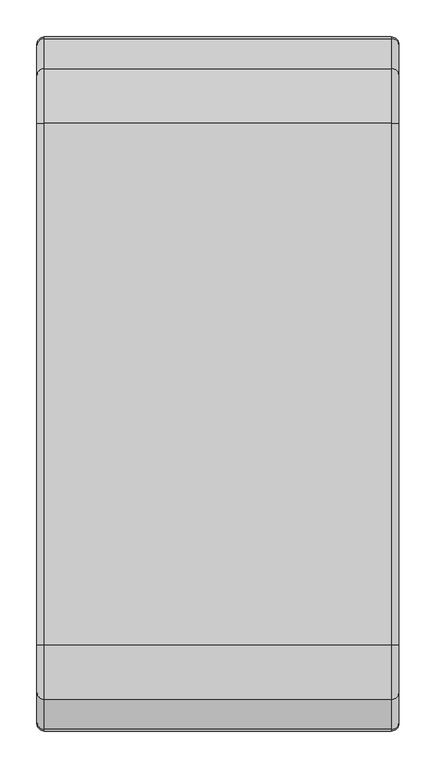
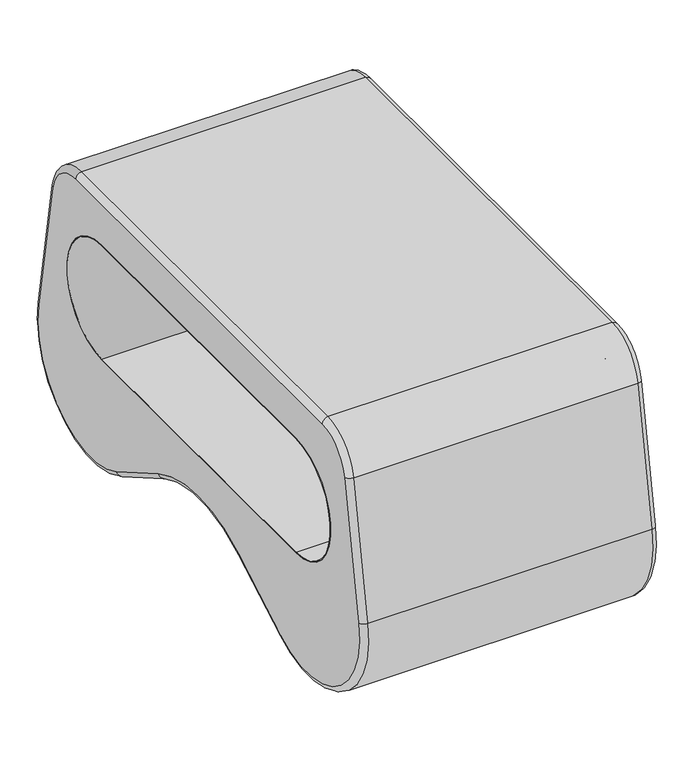
"""IFC4 building model written with IfcOpenShell, lengths in millimetres: furniture geometry."""

from ifc_helpers import new_model, si_unit, point, frame, origin, place, context, project, spatial, polyline, circle_curve, ellipse_curve, trimmed, source, transform, mapped, element, save
from ifc_brep_helpers import plane_surface, cylinder_surface, revolved_surface, advanced_brep


def furniture_2dca108f(model_context):
    return source(origin(), model_context, "Body", "AdvancedBrep", [
        advanced_brep(
        [(245.0, 417.1236557, 416.2871315), (245.0, 353.1111517, 470.0), (245.0, -353.1111517, 470.0), (245.0, -417.1236557, 416.2871315), (245.0, -457.721163, 186.0472267), (245.0, -235.0, 30.0961894), (245.0, -115.0, 99.3782217), (245.0, 115.0, 99.3782217), (245.0, 235.0, 30.0961894), (245.0, 457.721163, 186.0472267), (245.0, 278.278004, 200.0), (245.0, -278.278004, 200.0), (245.0, -278.278004, 400.0), (245.0, 278.278004, 400.0), (-245.0, 353.1111517, 470.0), (-245.0, 417.1236557, 416.2871315), (-245.0, 457.721163, 186.0472267), (-245.0, 235.0, 30.0961894), (-245.0, 115.0, 99.3782217), (-245.0, -115.0, 99.3782217), (-245.0, -235.0, 30.0961894), (-245.0, -457.721163, 186.0472267), (-245.0, -417.1236557, 416.2871315), (-245.0, -353.1111517, 470.0), (-245.0, 278.278004, 200.0), (-245.0, 278.278004, 400.0), (-245.0, -278.278004, 400.0), (-245.0, -278.278004, 200.0), (-235.0, 353.1111517, 480.0), (-235.0, -353.1111517, 480.0), (235.0, -353.1111517, 480.0), (235.0, 353.1111517, 480.0), (-235.0, -426.9717332, 418.0236133), (235.0000137, -426.9717332, 418.0236133), (-235.0, -467.5692405, 187.7837084), (235.0, -467.5692405, 187.7837084), (-235.0, -230.0, 21.4359354), (235.0000033, -230.0, 21.4359354), (-235.0, -110.0, 90.7179677), (235.0, -110.0, 90.7179677), (-235.0, 110.0, 90.7179677), (235.000004, 110.0, 90.7179677), (-235.0, 230.0, 21.4359354), (235.0, 230.0, 21.4359354), (-235.0, 467.5692405, 187.7837084), (235.0000035, 467.5692405, 187.7837084), (-235.0, 426.9717332, 418.0236133), (235.0000138, 426.9717332, 418.0236133), (244.0, 278.278004, 200.0), (-244.0, 278.278004, 200.0), (-244.0, -278.278004, 200.0), (244.0000012, -278.278004, 200.0), (-244.0, -278.278004, 400.0), (244.0000005, -278.278004, 400.0), (-244.0, 278.278004, 400.0), (244.0000012, 278.278004, 400.0)],
        [
            (0, 1, circle_curve(frame((245.0, 353.1111517, 405.0), z_axis=(1.0, 0.0, 0.0), x_axis=(0.0, 0.9848077530122095, 0.1736481776669226)), 65.0)),
            (1, 2),
            (2, 3, circle_curve(frame((245.0, -353.1111517, 405.0), z_axis=(1.0, 0.0, 0.0), x_axis=(0.0, 0.0, 1.0)), 65.0)),
            (3, 4),
            (4, 5, circle_curve(frame((245.0, -310.0, 160.0), z_axis=(1.0, 0.0, 0.0), x_axis=(0.0, -0.9848077530122084, 0.17364817766692853)), 150.0)),
            (5, 6),
            (6, 7, circle_curve(frame((245.0, 0.0, -99.8076211), z_axis=(-1.0, 0.0, 0.0), x_axis=(0.0, -0.4999999999999878, 0.8660254037844457)), 230.0)),
            (7, 8),
            (8, 9, circle_curve(frame((245.0, 310.0, 160.0), z_axis=(1.0, 0.0, 0.0), x_axis=(0.0, -0.5000000000000022, -0.8660254037844374)), 150.0)),
            (9, 0),
            (10, 11),
            (11, 12, circle_curve(frame((245.0, -278.278004, 300.0), z_axis=(-1.0, 0.0, 0.0), x_axis=(0.0, 1.0, 0.0)), 100.0)),
            (12, 13),
            (13, 10, circle_curve(frame((245.0, 278.278004, 300.0), z_axis=(-1.0, 0.0, 0.0), x_axis=(0.0, -1.0, 0.0)), 100.0)),
            (14, 15, circle_curve(frame((-245.0, 353.1111517, 405.0), z_axis=(-1.0, 0.0, 0.0), x_axis=(0.0, 0.9848077530122092, 0.17364817766692348)), 65.0)),
            (15, 16),
            (16, 17, circle_curve(frame((-245.0, 310.0, 160.0), z_axis=(-1.0, 0.0, 0.0), x_axis=(0.0, -0.5000000000000022, -0.8660254037844374)), 150.0)),
            (17, 18),
            (18, 19, circle_curve(frame((-245.0, 0.0, -99.8076211), z_axis=(1.0, 0.0, 0.0), x_axis=(0.0, -0.4999999999999878, 0.8660254037844457)), 230.0)),
            (19, 20),
            (20, 21, circle_curve(frame((-245.0, -310.0, 160.0), z_axis=(-1.0, 0.0, 0.0), x_axis=(0.0, -0.9848077530122084, 0.17364817766692853)), 150.0)),
            (21, 22),
            (22, 23, circle_curve(frame((-245.0, -353.1111517, 405.0), z_axis=(-1.0, 0.0, 0.0), x_axis=(0.0, 0.0, 1.0)), 65.0)),
            (23, 14),
            (24, 25, circle_curve(frame((-245.0, 278.278004, 300.0), z_axis=(1.0, 0.0, 0.0), x_axis=(0.0, -1.0, 0.0)), 100.0)),
            (25, 26),
            (26, 27, circle_curve(frame((-245.0, -278.278004, 300.0), z_axis=(1.0, 0.0, 0.0), x_axis=(0.0, 1.0, 0.0)), 100.0)),
            (27, 24),
            (28, 29),
            (29, 30),
            (30, 31),
            (31, 28),
            (29, 32, circle_curve(frame((-235.0, -353.1111517, 405.0), z_axis=(1.0, 0.0, 0.0), x_axis=(0.0, 1.0, 0.0)), 75.0)),
            (32, 33),
            (33, 30, circle_curve(frame((235.0, -353.1111517, 405.0), z_axis=(-1.0, 0.0, 0.0), x_axis=(0.0, 1.0, 0.0)), 75.0)),
            (32, 34),
            (34, 35),
            (35, 33),
            (34, 36, circle_curve(frame((-235.0, -310.0, 160.0), z_axis=(1.0, 0.0, 0.0), x_axis=(0.0, 1.0, 0.0)), 160.0)),
            (36, 37),
            (37, 35, circle_curve(frame((235.0, -310.0, 160.0), z_axis=(-1.0, 0.0, 0.0), x_axis=(0.0, 1.0, 0.0)), 160.0)),
            (36, 38),
            (38, 39),
            (39, 37),
            (38, 40, circle_curve(frame((-235.0, 0.0, -99.8076211), z_axis=(-1.0, 0.0, 0.0), x_axis=(0.0, -1.0, 0.0)), 220.0)),
            (40, 41),
            (41, 39, circle_curve(frame((235.0, 0.0, -99.8076211), z_axis=(1.0, 0.0, 0.0), x_axis=(0.0, -1.0, 0.0)), 220.0)),
            (40, 42),
            (42, 43),
            (43, 41),
            (42, 44, circle_curve(frame((-235.0, 310.0, 160.0), z_axis=(1.0, 0.0, 0.0), x_axis=(0.0, -1.0, 0.0)), 160.0)),
            (44, 45),
            (45, 43, circle_curve(frame((235.0, 310.0, 160.0), z_axis=(-1.0, 0.0, 0.0), x_axis=(0.0, -1.0, 0.0)), 160.0)),
            (44, 46),
            (46, 47),
            (47, 45),
            (46, 28, circle_curve(frame((-235.0, 353.1111517, 405.0), z_axis=(1.0, 0.0, 0.0), x_axis=(0.0, -1.0, 0.0)), 75.0)),
            (31, 47, circle_curve(frame((235.0, 353.1111517, 405.0), z_axis=(-1.0, 0.0, 0.0), x_axis=(0.0, -1.0, 0.0)), 75.0)),
            (10, 48),
            (48, 49),
            (49, 24),
            (27, 50),
            (50, 51),
            (51, 11),
            (26, 52),
            (52, 53),
            (53, 12),
            (25, 54),
            (54, 55),
            (55, 13),
            (14, 28, circle_curve(frame((-235.0, 353.1111517, 470.0), z_axis=(0.0, 1.0, 0.0), x_axis=(-1.0, 0.0, 0.0)), 10.0)),
            (46, 15, circle_curve(frame((-235.0, 417.1236557, 416.2871315), z_axis=(0.0, -0.17364817766692348, 0.9848077530122092), x_axis=(-1.0, 0.0, 0.0)), 10.0)),
            (23, 29, circle_curve(frame((-235.0, -353.1111517, 470.0), z_axis=(0.0, 1.0, 0.0), x_axis=(-1.0, 0.0, 0.0)), 10.0)),
            (22, 32, circle_curve(frame((-235.0, -417.1236557, 416.2871315), z_axis=(0.0, 0.17364817766692897, 0.9848077530122084), x_axis=(-1.0, 0.0, 0.0)), 10.0)),
            (21, 34, circle_curve(frame((-235.0, -457.721163, 186.0472267), z_axis=(0.0, 0.1736481776669289, 0.9848077530122084), x_axis=(-1.0, 0.0, 0.0)), 10.0)),
            (20, 36, circle_curve(frame((-235.0, -235.0, 30.0961894), z_axis=(0.0, -0.8660254037844488, -0.4999999999999824), x_axis=(-1.0, 0.0, 0.0)), 10.0)),
            (19, 38, circle_curve(frame((-235.0, -115.0, 99.3782217), z_axis=(0.0, -0.8660254037844457, -0.4999999999999879), x_axis=(-1.0, 0.0, 0.0)), 10.0)),
            (18, 40, circle_curve(frame((-235.0, 115.0, 99.3782217), z_axis=(0.0, -0.8660254037844375, 0.500000000000002), x_axis=(-1.0, 0.0, 0.0)), 10.0)),
            (17, 42, circle_curve(frame((-235.0, 235.0, 30.0961894), z_axis=(0.0, -0.8660254037844374, 0.5000000000000023), x_axis=(-1.0, 0.0, 0.0)), 10.0)),
            (16, 44, circle_curve(frame((-235.0, 457.721163, 186.0472267), z_axis=(0.0, 0.1736481776669226, -0.9848077530122095), x_axis=(-1.0, 0.0, 0.0)), 10.0)),
            (31, 1, circle_curve(frame((235.0, 353.1111517, 470.0), z_axis=(0.0, 1.0, 0.0), x_axis=(1.0, 0.0, 0.0)), 10.0)),
            (0, 47, circle_curve(frame((235.0, 417.1236557, 416.2871315), z_axis=(0.0, -0.1736481776669226, 0.9848077530122095), x_axis=(1.0, 0.0, 0.0)), 10.0)),
            (30, 2, circle_curve(frame((235.0, -353.1111517, 470.0), z_axis=(0.0, 1.0, 0.0), x_axis=(1.0, 0.0, 0.0)), 10.0)),
            (33, 3, circle_curve(frame((235.0, -417.1236557, 416.2871315), z_axis=(0.0, 0.1736481776669292, 0.9848077530122084), x_axis=(1.0, 0.0, 0.0)), 10.0)),
            (35, 4, circle_curve(frame((235.0, -457.721163, 186.0472267), z_axis=(0.0, 0.1736481776669289, 0.9848077530122084), x_axis=(1.0, 0.0, 0.0)), 10.0)),
            (37, 5, circle_curve(frame((235.0, -235.0, 30.0961894), z_axis=(0.0, -0.8660254037844488, -0.4999999999999824), x_axis=(1.0, 0.0, 0.0)), 10.0)),
            (39, 6, circle_curve(frame((235.0, -115.0, 99.3782217), z_axis=(0.0, -0.8660254037844457, -0.4999999999999879), x_axis=(1.0, 0.0, 0.0)), 10.0)),
            (41, 7, circle_curve(frame((235.0, 115.0, 99.3782217), z_axis=(0.0, -0.8660254037844375, 0.5000000000000022), x_axis=(1.0, 0.0, 0.0)), 10.0)),
            (43, 8, circle_curve(frame((235.0, 235.0, 30.0961894), z_axis=(0.0, -0.8660254037844375, 0.5000000000000022), x_axis=(1.0, 0.0, 0.0)), 10.0)),
            (45, 9, circle_curve(frame((235.0, 457.721163, 186.0472267), z_axis=(0.0, 0.1736481776669226, -0.9848077530122095), x_axis=(1.0, 0.0, 0.0)), 10.0)),
        ],
        [
            plane_surface(frame((245.0, 0.0, 480.0), z_axis=(1.0, 0.0, 0.0), x_axis=(0.0, -1.0, 0.0))),
            plane_surface(frame((-245.0, 0.0, 480.0), z_axis=(-1.0, 0.0, 0.0), x_axis=(0.0, 1.0, 0.0))),
            plane_surface(frame((245.0, 353.1111517, 480.0), z_axis=(0.0, 0.0, 1.0), x_axis=(-1.0, 0.0, 0.0))),
            cylinder_surface(frame((-245.0, -353.1111517, 405.0), z_axis=(1.0, 0.0, 0.0), x_axis=(0.0, 1.0, 0.0)), 75.0),
            plane_surface(frame((245.0, -426.9717332, 418.0236133), z_axis=(0.0, -0.9848077530122084, 0.17364817766692886), x_axis=(-1.0, 0.0, 0.0))),
            cylinder_surface(frame((-245.0, -310.0, 160.0), z_axis=(1.0, 0.0, 0.0), x_axis=(0.0, 1.0, 0.0)), 160.0),
            plane_surface(frame((245.0, -230.0, 21.4359354), z_axis=(0.0, 0.4999999999999879, -0.8660254037844457), x_axis=(-1.0, 0.0, 0.0))),
            revolved_surface(polyline([(-235.0, -220.0, -99.8076211), (235.000004, -220.0, -99.8076211)]), (-245.0, 0.0, -99.8076211), (-1.0, 0.0, 0.0)),
            plane_surface(frame((245.0, 110.0, 90.7179677), z_axis=(0.0, -0.5000000000000021, -0.8660254037844375), x_axis=(-1.0, 0.0, 0.0))),
            cylinder_surface(frame((-245.0, 310.0, 160.0), z_axis=(1.0, 0.0, 0.0), x_axis=(0.0, -1.0, 0.0)), 160.0),
            plane_surface(frame((245.0, 467.5692405, 187.7837084), z_axis=(0.0, 0.9848077530122084, 0.17364817766692872), x_axis=(-1.0, 0.0, 0.0))),
            cylinder_surface(frame((-245.0, 353.1111517, 405.0), z_axis=(1.0, 0.0, 0.0), x_axis=(0.0, -1.0, 0.0)), 75.0),
            plane_surface(frame((245.0, 278.278004, 200.0), z_axis=(0.0, 0.0, 1.0), x_axis=(-1.0, 0.0, 0.0))),
            revolved_surface(polyline([(-245.0, -178.278004, 300.0), (245.0, -178.278004, 300.0)]), (0.0, -278.278004, 300.0), (-1.0, 0.0, 0.0)),
            plane_surface(frame((245.0, -278.278004, 400.0), z_axis=(0.0, 0.0, -1.0), x_axis=(-1.0, 0.0, 0.0))),
            revolved_surface(polyline([(-245.0, 178.278004, 300.0), (245.0, 178.278004, 300.0)]), (0.0, 278.278004, 300.0), (-1.0, 0.0, 0.0)),
            revolved_surface(trimmed(ellipse_curve(frame((-235.0, 417.1236557, 416.2871315), z_axis=(0.0, 0.17364817766692348, -0.9848077530122092), x_axis=(-1.0, 0.0, 0.0)), 10.0, 10.0), [point((-245.0, 417.1236557, 416.2871315))], [point((-235.0, 426.9717332, 418.0236133))], True, "CARTESIAN"), (0.0, 353.1111517, 405.0), (1.0, 0.0, 0.0)),
            cylinder_surface(frame((-235.0, 353.1111517, 470.0), z_axis=(0.0, -1.0, 0.0), x_axis=(-1.0, 0.0, 0.0)), 10.0),
            revolved_surface(trimmed(ellipse_curve(frame((-235.0, -353.1111517, 470.0), z_axis=(0.0, 1.0, 0.0), x_axis=(-1.0, 0.0, 0.0)), 10.0, 10.0), [point((-245.0, -353.1111517, 470.0))], [point((-235.0, -353.1111517, 480.0))], True, "CARTESIAN"), (0.0, -353.1111517, 405.0), (1.0, 0.0, 0.0)),
            cylinder_surface(frame((-235.0, -417.1236557, 416.2871315), z_axis=(0.0, -0.1736481776669289, -0.9848077530122084), x_axis=(-1.0, 0.0, 0.0)), 10.0),
            revolved_surface(trimmed(ellipse_curve(frame((-235.0, -457.721163, 186.0472267), z_axis=(0.0, 0.17364817766692855, 0.9848077530122084), x_axis=(-1.0, 0.0, 0.0)), 10.0, 10.0), [point((-245.0, -457.721163, 186.0472267))], [point((-235.0, -467.5692405, 187.7837084))], True, "CARTESIAN"), (0.0, -310.0, 160.0), (1.0, 0.0, 0.0)),
            cylinder_surface(frame((-235.0, -235.0, 30.0961894), z_axis=(0.0, 0.8660254037844457, 0.4999999999999879), x_axis=(-1.0, 0.0, 0.0)), 10.0),
            revolved_surface(trimmed(ellipse_curve(frame((-235.0, -115.0, 99.3782217), z_axis=(0.0, -0.8660254037844457, -0.4999999999999878), x_axis=(-1.0, 0.0, 0.0)), 10.0, 10.0), [point((-245.0, -115.0, 99.3782217))], [point((-235.0, -110.0, 90.7179677))], True, "CARTESIAN"), (0.0, 0.0, -99.8076211), (-1.0, 0.0, 0.0)),
            cylinder_surface(frame((-235.0, 115.0, 99.3782217), z_axis=(0.0, 0.8660254037844374, -0.5000000000000023), x_axis=(-1.0, 0.0, 0.0)), 10.0),
            revolved_surface(trimmed(ellipse_curve(frame((-235.0, 235.0, 30.0961894), z_axis=(0.0, -0.8660254037844374, 0.5000000000000022), x_axis=(-1.0, 0.0, 0.0)), 10.0, 10.0), [point((-245.0, 235.0, 30.0961894))], [point((-235.0, 230.0, 21.4359354))], True, "CARTESIAN"), (0.0, 310.0, 160.0), (1.0, 0.0, 0.0)),
            cylinder_surface(frame((-235.0, 457.721163, 186.0472267), z_axis=(0.0, -0.17364817766692864, 0.9848077530122085), x_axis=(-1.0, 0.0, 0.0)), 10.0),
            revolved_surface(trimmed(ellipse_curve(frame((235.0, 417.1236557, 416.2871315), z_axis=(0.0, 0.1736481776669226, -0.9848077530122095), x_axis=(1.0, 0.0, 0.0)), 10.0, 10.0), [point((235.0, 426.9717332, 418.0236133))], [point((245.0, 417.1236557, 416.2871315))], True, "CARTESIAN"), (0.0, 353.1111517, 405.0), (1.0, 0.0, 0.0)),
            cylinder_surface(frame((235.0, 353.1111517, 470.0), z_axis=(0.0, -1.0, 0.0), x_axis=(1.0, 0.0, 0.0)), 10.0),
            revolved_surface(trimmed(ellipse_curve(frame((235.0, -353.1111517, 470.0), z_axis=(0.0, 1.0, 0.0), x_axis=(1.0, 0.0, 0.0)), 10.0, 10.0), [point((235.0, -353.1111517, 480.0))], [point((245.0, -353.1111517, 470.0))], True, "CARTESIAN"), (0.0, -353.1111517, 405.0), (1.0, 0.0, 0.0)),
            cylinder_surface(frame((235.0, -417.1236557, 416.2871315), z_axis=(0.0, -0.1736481776669289, -0.9848077530122084), x_axis=(1.0, 0.0, 0.0)), 10.0),
            revolved_surface(trimmed(ellipse_curve(frame((235.0, -457.721163, 186.0472267), z_axis=(0.0, 0.17364817766692855, 0.9848077530122084), x_axis=(1.0, 0.0, 0.0)), 10.0, 10.0), [point((235.0, -467.5692405, 187.7837084))], [point((245.0, -457.721163, 186.0472267))], True, "CARTESIAN"), (0.0, -310.0, 160.0), (1.0, 0.0, 0.0)),
            cylinder_surface(frame((235.0, -235.0, 30.0961894), z_axis=(0.0, 0.8660254037844457, 0.4999999999999879), x_axis=(1.0, 0.0, 0.0)), 10.0),
            revolved_surface(trimmed(ellipse_curve(frame((235.0, -115.0, 99.3782217), z_axis=(0.0, -0.8660254037844457, -0.4999999999999878), x_axis=(1.0, 0.0, 0.0)), 10.0, 10.0), [point((235.0, -110.0, 90.7179677))], [point((245.0, -115.0, 99.3782217))], True, "CARTESIAN"), (0.0, 0.0, -99.8076211), (-1.0, 0.0, 0.0)),
            cylinder_surface(frame((235.0, 115.0, 99.3782217), z_axis=(0.0, 0.8660254037844375, -0.5000000000000022), x_axis=(1.0, 0.0, 0.0)), 10.0),
            revolved_surface(trimmed(ellipse_curve(frame((235.0, 235.0, 30.0961894), z_axis=(0.0, -0.8660254037844374, 0.5000000000000022), x_axis=(1.0, 0.0, 0.0)), 10.0, 10.0), [point((235.0, 230.0, 21.4359354))], [point((245.0, 235.0, 30.0961894))], True, "CARTESIAN"), (0.0, 310.0, 160.0), (1.0, 0.0, 0.0)),
            cylinder_surface(frame((235.0, 457.721163, 186.0472267), z_axis=(0.0, -0.17364817766692878, 0.9848077530122084), x_axis=(1.0, 0.0, 0.0)), 10.0),
        ],
        [
            (0, [[1, 2, 3, 4, 5, 6, 7, 8, 9, 10], [11, 12, 13, 14]]),
            (1, [[15, 16, 17, 18, 19, 20, 21, 22, 23, 24], [25, 26, 27, 28]]),
            (2, [[29, 30, 31, 32]]),
            (3, [[33, 34, 35, -30]]),
            (4, [[36, 37, 38, -34]]),
            (5, [[39, 40, 41, -37]]),
            (6, [[42, 43, 44, -40]]),
            (7, [[45, 46, 47, -43]]),
            (8, [[48, 49, 50, -46]]),
            (9, [[51, 52, 53, -49]]),
            (10, [[54, 55, 56, -52]]),
            (11, [[57, -32, 58, -55]]),
            (12, [[-11, 59, 60, 61, -28, 62, 63, 64]]),
            (13, [[-12, -64, -63, -62, -27, 65, 66, 67]]),
            (14, [[-13, -67, -66, -65, -26, 68, 69, 70]]),
            (15, [[-14, -70, -69, -68, -25, -61, -60, -59]]),
            (16, [[71, -57, 72, -15]]),
            (17, [[-71, -24, 73, -29]]),
            (18, [[-73, -23, 74, -33]]),
            (19, [[-74, -22, 75, -36]]),
            (20, [[-75, -21, 76, -39]]),
            (21, [[-76, -20, 77, -42]]),
            (22, [[-77, -19, 78, -45]]),
            (23, [[-78, -18, 79, -48]]),
            (24, [[-79, -17, 80, -51]]),
            (25, [[-72, -54, -80, -16]]),
            (26, [[81, -1, 82, -58]]),
            (27, [[-81, -31, 83, -2]]),
            (28, [[-83, -35, 84, -3]]),
            (29, [[-84, -38, 85, -4]]),
            (30, [[-85, -41, 86, -5]]),
            (31, [[-86, -44, 87, -6]]),
            (32, [[-87, -47, 88, -7]]),
            (33, [[-88, -50, 89, -8]]),
            (34, [[-89, -53, 90, -9]]),
            (35, [[-82, -10, -90, -56]]),
        ],
    ),
        advanced_brep(
        [(-244.0, -278.278004, 200.0), (-244.0, 278.278004, 200.0), (244.0, 278.278004, 200.0), (244.0, -278.278004, 200.0), (-244.0, 278.278004, 400.0), (244.0000012, 278.278004, 400.0), (-244.0, -278.278004, 400.0), (244.0000012, -278.278004, 400.0), (245.0, 278.278004, 399.0), (-245.0, 278.278004, 399.0), (-245.0, 278.278004, 201.0), (245.0, 278.278004, 201.0), (-245.0, -278.278004, 201.0), (245.0, -278.278004, 201.0), (-245.0, -278.278004, 399.0), (245.0, -278.278004, 399.0)],
        [
            (0, 1),
            (1, 2),
            (2, 3),
            (3, 0),
            (1, 4, circle_curve(frame((-244.0, 278.278004, 300.0), z_axis=(1.0, 0.0, 0.0), x_axis=(0.0, -1.0, 0.0)), 100.0)),
            (4, 5),
            (5, 2, circle_curve(frame((244.0, 278.278004, 300.0), z_axis=(-1.0, 0.0, 0.0), x_axis=(0.0, -1.0, 0.0)), 100.0)),
            (4, 6),
            (6, 7),
            (7, 5),
            (6, 0, circle_curve(frame((-244.0, -278.278004, 300.0), z_axis=(1.0, 0.0, 0.0), x_axis=(0.0, 1.0, 0.0)), 100.0)),
            (3, 7, circle_curve(frame((244.0, -278.278004, 300.0), z_axis=(-1.0, 0.0, 0.0), x_axis=(0.0, 1.0, 0.0)), 100.0)),
            (8, 9),
            (9, 10, circle_curve(frame((-245.0, 278.278004, 300.0), z_axis=(-1.0, 0.0, 0.0), x_axis=(0.0, -1.0, 0.0)), 99.0)),
            (10, 11),
            (11, 8, circle_curve(frame((245.0, 278.278004, 300.0), z_axis=(1.0, 0.0, 0.0), x_axis=(0.0, -1.0, 0.0)), 99.0)),
            (10, 12),
            (12, 13),
            (13, 11),
            (12, 14, circle_curve(frame((-245.0, -278.278004, 300.0), z_axis=(-1.0, 0.0, 0.0), x_axis=(0.0, 1.0, 0.0)), 99.0)),
            (14, 15),
            (15, 13, circle_curve(frame((245.0, -278.278004, 300.0), z_axis=(1.0, 0.0, 0.0), x_axis=(0.0, 1.0, 0.0)), 99.0)),
            (8, 15),
            (14, 9),
            (12, 0, circle_curve(frame((-244.0, -278.278004, 201.0), z_axis=(0.0, -1.0, 0.0), x_axis=(-1.0, 0.0, 0.0)), 1.0)),
            (6, 14, circle_curve(frame((-244.0, -278.278004, 399.0), z_axis=(0.0, -1.0, 0.0), x_axis=(-1.0, 0.0, 0.0)), 1.0)),
            (10, 1, circle_curve(frame((-244.0, 278.278004, 201.0), z_axis=(0.0, -1.0, 0.0), x_axis=(-1.0, 0.0, 0.0)), 1.0)),
            (9, 4, circle_curve(frame((-244.0, 278.278004, 399.0), z_axis=(0.0, 1.0, 0.0), x_axis=(-1.0, 0.0, 0.0)), 1.0)),
            (3, 13, circle_curve(frame((244.0, -278.278004, 201.0), z_axis=(0.0, -1.0, 0.0), x_axis=(1.0, 0.0, 0.0)), 1.0)),
            (15, 7, circle_curve(frame((244.0, -278.278004, 399.0), z_axis=(0.0, -1.0, 0.0), x_axis=(1.0, 0.0, 0.0)), 1.0)),
            (2, 11, circle_curve(frame((244.0, 278.278004, 201.0), z_axis=(0.0, -1.0, 0.0), x_axis=(1.0, 0.0, 0.0)), 1.0)),
            (5, 8, circle_curve(frame((244.0, 278.278004, 399.0), z_axis=(0.0, 1.0, 0.0), x_axis=(1.0, 0.0, 0.0)), 1.0)),
        ],
        [
            plane_surface(frame((245.0, -278.278004, 200.0), z_axis=(0.0, 0.0, -1.0), x_axis=(-1.0, 0.0, 0.0))),
            cylinder_surface(frame((-245.0, 278.278004, 300.0), z_axis=(1.0, 0.0, 0.0), x_axis=(0.0, -1.0, 0.0)), 100.0),
            plane_surface(frame((245.0, 278.278004, 400.0), z_axis=(0.0, 0.0, 1.0), x_axis=(-1.0, 0.0, 0.0))),
            cylinder_surface(frame((-245.0, -278.278004, 300.0), z_axis=(1.0, 0.0, 0.0), x_axis=(0.0, 1.0, 0.0)), 100.0),
            revolved_surface(polyline([(-245.0, 179.278004, 300.0), (245.0, 179.278004, 300.0)]), (0.0, 278.278004, 300.0), (-1.0, 0.0, 0.0)),
            plane_surface(frame((245.0, 278.278004, 201.0), z_axis=(0.0, 0.0, 1.0), x_axis=(-1.0, 0.0, 0.0))),
            revolved_surface(polyline([(-245.0, -179.278004, 300.0), (245.0, -179.278004, 300.0)]), (0.0, -278.278004, 300.0), (-1.0, 0.0, 0.0)),
            plane_surface(frame((245.0, -278.278004, 399.0), z_axis=(0.0, 0.0, -1.0), x_axis=(-1.0, 0.0, 0.0))),
            revolved_surface(trimmed(ellipse_curve(frame((-244.0, -278.278004, 399.0), z_axis=(0.0, 1.0, 0.0), x_axis=(-1.0, 0.0, 0.0)), 1.0, 1.0), [point((-245.0, -278.278004, 399.0))], [point((-244.0, -278.278004, 400.0))], True, "CARTESIAN"), (0.0, -278.278004, 300.0), (1.0, 0.0, 0.0)),
            cylinder_surface(frame((-244.0, -278.278004, 201.0), z_axis=(0.0, 1.0, 0.0), x_axis=(-1.0, 0.0, 0.0)), 1.0),
            revolved_surface(trimmed(ellipse_curve(frame((-244.0, 278.278004, 201.0), z_axis=(0.0, -1.0, 0.0), x_axis=(-1.0, 0.0, 0.0)), 1.0, 1.0), [point((-245.0, 278.278004, 201.0))], [point((-244.0, 278.278004, 200.0))], True, "CARTESIAN"), (0.0, 278.278004, 300.0), (1.0, 0.0, 0.0)),
            cylinder_surface(frame((-244.0, 278.278004, 399.0), z_axis=(0.0, -1.0, 0.0), x_axis=(-1.0, 0.0, 0.0)), 1.0),
            revolved_surface(trimmed(ellipse_curve(frame((244.0, -278.278004, 399.0), z_axis=(0.0, 1.0, 0.0), x_axis=(1.0, 0.0, 0.0)), 1.0, 1.0), [point((244.0, -278.278004, 400.0))], [point((245.0, -278.278004, 399.0))], True, "CARTESIAN"), (0.0, -278.278004, 300.0), (1.0, 0.0, 0.0)),
            cylinder_surface(frame((244.0, -278.278004, 201.0), z_axis=(0.0, 1.0, 0.0), x_axis=(1.0, 0.0, 0.0)), 1.0),
            revolved_surface(trimmed(ellipse_curve(frame((244.0, 278.278004, 201.0), z_axis=(0.0, -1.0, 0.0), x_axis=(1.0, 0.0, 0.0)), 1.0, 1.0), [point((244.0, 278.278004, 200.0))], [point((245.0, 278.278004, 201.0))], True, "CARTESIAN"), (0.0, 278.278004, 300.0), (1.0, 0.0, 0.0)),
            cylinder_surface(frame((244.0, 278.278004, 399.0), z_axis=(0.0, -1.0, 0.0), x_axis=(1.0, 0.0, 0.0)), 1.0),
        ],
        [
            (0, [[1, 2, 3, 4]]),
            (1, [[5, 6, 7, -2]]),
            (2, [[8, 9, 10, -6]]),
            (3, [[11, -4, 12, -9]]),
            (4, [[13, 14, 15, 16]]),
            (5, [[-15, 17, 18, 19]]),
            (6, [[-18, 20, 21, 22]]),
            (7, [[-13, 23, -21, 24]]),
            (8, [[25, -11, 26, -20]]),
            (9, [[-25, -17, 27, -1]]),
            (10, [[-27, -14, 28, -5]]),
            (11, [[-26, -8, -28, -24]]),
            (12, [[29, -22, 30, -12]]),
            (13, [[-29, -3, 31, -19]]),
            (14, [[-31, -7, 32, -16]]),
            (15, [[-30, -23, -32, -10]]),
        ],
    ),
    ])


if __name__ == "__main__":
    model = new_model("IFC4")
    model_context = context("Model", 3, world=origin())
    ifc_project = project(units=[si_unit("LENGTHUNIT", "METRE", prefix="MILLI")], contexts=[model_context])
    site = spatial("IfcSite", under=ifc_project)
    building = spatial("IfcBuilding", under=site)
    placement = place(None, origin())
    furniture_shape = furniture_2dca108f(model_context)
    element("IfcFurniture", 1, at=placement, inside=building, context=model_context, shape_type="MappedRepresentation", body=[
        mapped(furniture_shape, transform((0.0, 0.0, 0.0), x_axis=(1.0, 0.0, 0.0), y_axis=(0.0, 1.0, 0.0), z_axis=(0.0, 0.0, 1.0))),
    ])
    save(model, "model.ifc")

# Revit data of these elements
# Type
#   Default Elevation = 0
